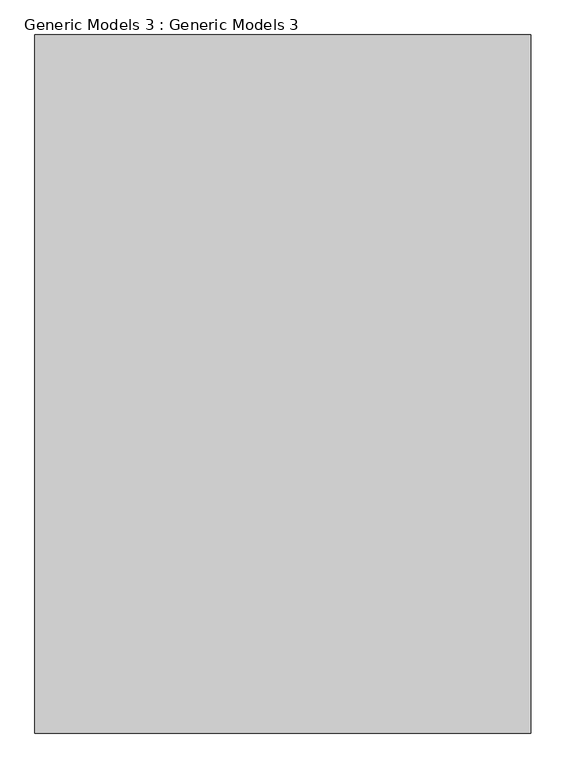
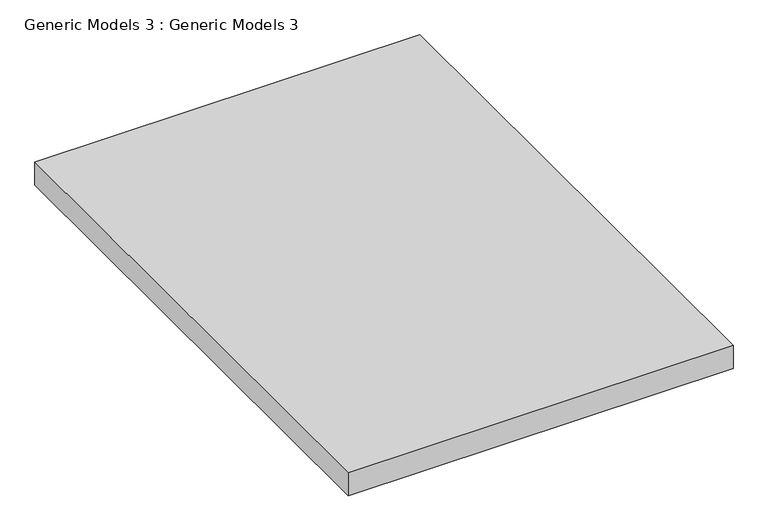
"""IFC4 building model written with IfcOpenShell, lengths in millimetres: proxy geometry, Generic Models 3 : Generic Models 3."""

from ifc_helpers import new_model, si_unit, frame, origin, place, context, project, spatial, polyline, outline, extrude, source, transform, mapped, element, save


def generic_models_3_generic_models_3_5fb3f9a6(model_context):
    return source(origin(), model_context, "Body", "SweptSolid", [
        extrude(outline(polyline([(-1718.5120831, -8122.2264512), (-6594.799579, -8122.2264512), (-6594.799579, -1254.7945627), (-1718.5120831, -1254.7945627), (-1718.5120831, -8122.2264512)])), frame((0.0, 0.0, 9015.3547159), z_axis=(0.0, 0.0, 1.0), x_axis=(1.0, 0.0, 0.0)), (0.0, 0.0, 1.0), 304.8),
    ])


if __name__ == "__main__":
    model = new_model("IFC4")
    model_context = context("Model", 3, world=origin())
    ifc_project = project(units=[si_unit("LENGTHUNIT", "METRE", prefix="MILLI")], contexts=[model_context])
    site = spatial("IfcSite", under=ifc_project)
    building = spatial("IfcBuilding", under=site)
    placement = place(None, origin())
    generic_models_3_generic_models_3_shape = generic_models_3_generic_models_3_5fb3f9a6(model_context)
    element("IfcBuildingElementProxy", 1, Name="Generic Models 3 : Generic Models 3", ObjectType="Generic Models 3 : Generic Models 3", at=placement, inside=building, context=model_context, shape_type="MappedRepresentation", body=[
        mapped(generic_models_3_generic_models_3_shape, transform((0.0, 0.0, 0.0), x_axis=(1.0, 0.0, 0.0), y_axis=(0.0, 1.0, 0.0), z_axis=(0.0, 0.0, 1.0))),
    ])
    save(model, "model.ifc")
